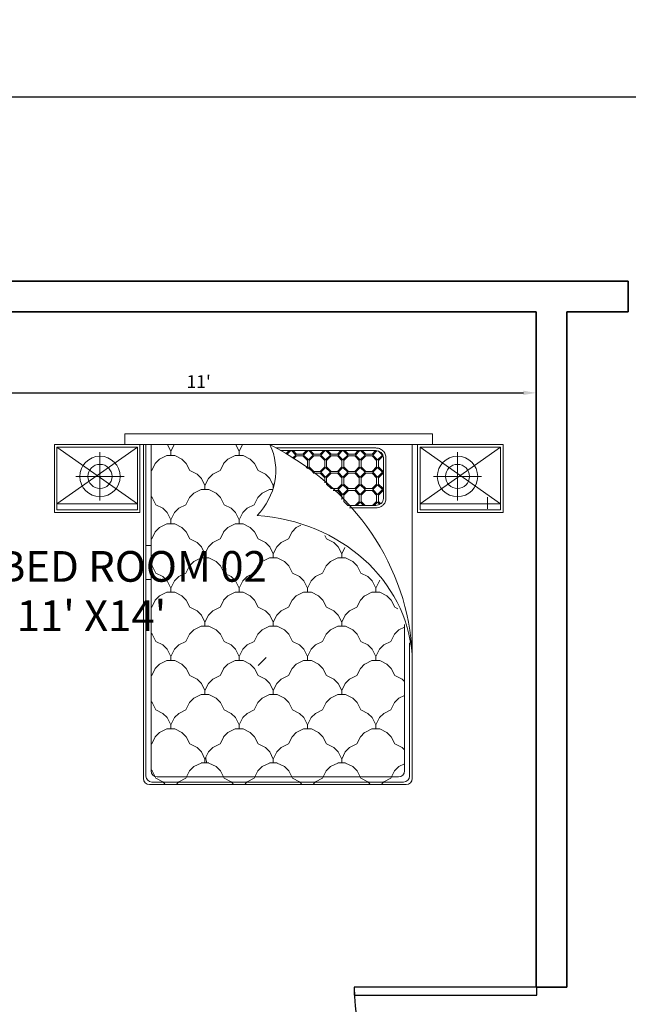
# Model space of a CAD drawing. Units: inches. Extents: x 2025 to 2528, y 1525 to 2336.
# Tile 7 of 18: x 2106 to 2225, y 1974 to 2167. Entities that reach past the tile are written whole.
import ezdxf

# ---------------------------------------------------------------- set-up
doc = ezdxf.new("R2010")
doc.units = ezdxf.units.IN
for name, color, linetype, lineweight in [('A-ANNO-DIMS', 2, 'Continuous', 18), ('A-AREA-IDEN', 7, 'Continuous', 25), ('A-DOOR', 3, 'Continuous', 25), ('A-FURN', 8, 'Continuous', 18), ('A-WALL', 7, 'Continuous', 35)]:
    doc.layers.add(name, color=color, linetype=linetype, lineweight=lineweight)
doc.styles.get("Standard").update_dxf_attribs({"font": 'arial.ttf'})
doc.dimstyles.new('Copy of ISO-25', dxfattribs={"dimtxt": 2.5, "dimasz": 2.5, "dimexe": 1.25, "dimexo": 0.625, "dimtad": 1, "dimdec": 1, "dimlunit": 4, "dimtxsty": 'Standard', "dimcen": 2.5, "dimadec": 0, "dimazin": 0, "dimtfac": 1, "dimtdec": 1, "dimtmove": 0, "dimatfit": 3, "dimfxl": 1, "dimarcsym": 0})

# ---------------------------------------------------------------- blocks, each defined once
blk = doc.blocks.new('*U5')
for p, q in [((0, 0), (0, -6)), ((-40, 0), (-40, -6))]:
    blk.add_line(p, q)
blk.add_lwpolyline([(0, 0), (0, 40), (-1.75, 40), (-1.75, 0)], close=True)
blk.add_arc((0, 0), 40, 90, 180)
blk = doc.blocks.new('*D12')
at = {"layer": 'A-ANNO-DIMS', "color": 0, "lineweight": -2, "transparency": 16777216}
for p, q in [((2075.01, 2108.79), (2075.01, 2092.35)), ((2207.01, 2108.79), (2207.01, 2092.35)), ((2077.51, 2093.6), (2204.51, 2093.6))]:
    blk.add_line(p, q, dxfattribs=at)
at = {"layer": 'A-ANNO-DIMS', "color": 0, "transparency": 16777216}
for points in [[(2077.51, 2094.02), (2077.51, 2093.19), (2075.01, 2093.6)], [(2204.51, 2094.02), (2204.51, 2093.19), (2207.01, 2093.6)]]:
    blk.add_solid(points, dxfattribs=at)
at = {"layer": 'Defpoints', "color": 0, "transparency": 16777216}
for p in [(2075.01, 2109.41), (2207.01, 2109.41), (2207.01, 2093.6)]:
    blk.add_point(p, dxfattribs=at)
at = {"layer": 'A-ANNO-DIMS', "color": 0, "transparency": 16777216, "insert": (2141.01, 2095.48), "char_height": 2.5, "attachment_point": 5}
blk.add_mtext("11'", dxfattribs=at)
blk = doc.blocks.new('A$C029D5C69')
for p, q in [((0.4164, 2.0693), (0.4164, 2.0066)), ((2.2315, 2.0693), (0.4164, 2.0693)), ((2.2315, 2.0066), (2.2315, 2.0693)), ((0, 1.606), (0, 2.0066)), ((0, 2.0066), (0.505, 2.0066)), ((0.0151, 1.6211), (0.0151, 1.9915)), ((0.0151, 1.9915), (0.4899, 1.9915)), ((0.4164, 2.0066), (2.2315, 2.0066)), ((0.4899, 1.9915), (0.4899, 1.6211)), ((0.505, 2.0066), (0.505, 1.606)), ((0.5252, 0.0351), (0.5252, 2.0066)), ((0.5403, 0.0502), (0.5403, 2.0066)), ((0.5706, 0.0805), (0.5706, 2.0066)), ((0.6869, 1.966), (0.6666, 2.0066)), ((0.7072, 2.0066), (0.6869, 1.966)), ((1.0902, 1.966), (1.0699, 2.0066)), ((1.1106, 2.0066), (1.0902, 1.966)), ((1.8954, 1.9865), (1.3081, 1.9865)), ((2.1114, 2.0087), (2.1114, 0.0351)), ((2.6479, 2.0066), (2.1429, 2.0066)), ((2.1429, 2.0066), (2.1429, 1.606)), ((2.6328, 1.9915), (2.158, 1.9915)), ((2.158, 1.9915), (2.158, 1.6211)), ((2.6328, 1.6211), (2.6328, 1.9915)), ((2.6479, 1.606), (2.6479, 2.0066)), ((0.2689, 1.9609), (0.2689, 1.6764)), ((0.621, 1.9213), (0.5955, 1.8958)), ((0.6634, 1.9425), (0.621, 1.9213)), ((0.6634, 1.9425), (0.621, 1.9213)), ((0.6869, 1.9425), (0.6634, 1.9425)), ((0.6869, 1.9425), (0.6869, 1.966)), ((0.6869, 1.9425), (0.6869, 1.966)), ((0.6869, 1.9425), (0.7104, 1.9425)), ((0.7528, 1.9213), (0.7104, 1.9425)), ((0.7528, 1.9213), (0.7104, 1.9425)), ((0.7783, 1.8958), (0.7528, 1.9213)), ((1.0243, 1.9213), (0.9988, 1.8958)), ((1.0668, 1.9425), (1.0244, 1.9213)), ((1.0668, 1.9425), (1.0244, 1.9213)), ((1.0902, 1.9425), (1.0668, 1.9425)), ((1.0902, 1.9425), (1.0902, 1.966)), ((1.0902, 1.9425), (1.0902, 1.966)), ((1.0902, 1.9425), (1.1137, 1.9425)), ((1.1561, 1.9213), (1.1137, 1.9425)), ((1.1561, 1.9213), (1.1137, 1.9425)), ((1.1816, 1.8958), (1.1561, 1.9213)), ((1.8954, 1.9713), (1.3339, 1.9713)), ((1.3849, 1.9713), (1.3656, 1.952)), ((1.3945, 1.9713), (1.3714, 1.9483)), ((1.4249, 1.945), (1.3986, 1.9713)), ((1.4249, 1.945), (1.4059, 1.926)), ((1.4288, 1.9507), (1.4081, 1.9713)), ((1.4288, 1.9394), (1.4116, 1.9222)), ((1.4476, 1.9507), (1.4288, 1.9507)), ((1.4288, 1.9393), (1.4476, 1.9393)), ((1.4476, 1.9507), (1.4664, 1.9507)), ((1.4664, 1.9393), (1.4476, 1.9393)), ((1.487, 1.9713), (1.4664, 1.9507)), ((1.493, 1.9128), (1.4664, 1.9394)), ((1.4966, 1.9713), (1.4703, 1.945)), ((1.4986, 1.9167), (1.4703, 1.945)), ((1.527, 1.945), (1.4986, 1.9167)), ((1.527, 1.945), (1.5007, 1.9713)), ((1.5309, 1.9394), (1.5043, 1.9128)), ((1.5309, 1.9507), (1.5102, 1.9713)), ((1.5497, 1.9507), (1.5309, 1.9507)), ((1.5309, 1.9393), (1.5497, 1.9393)), ((1.5497, 1.9507), (1.5685, 1.9507)), ((1.5685, 1.9393), (1.5497, 1.9393)), ((1.5891, 1.9713), (1.5685, 1.9507)), ((1.595, 1.9128), (1.5685, 1.9394)), ((1.5987, 1.9713), (1.5724, 1.945)), ((1.6007, 1.9167), (1.5724, 1.945)), ((1.6291, 1.945), (1.6007, 1.9167)), ((1.6291, 1.945), (1.6028, 1.9713)), ((1.633, 1.9394), (1.6064, 1.9128)), ((1.633, 1.9507), (1.6123, 1.9713)), ((1.6518, 1.9507), (1.633, 1.9507)), ((1.633, 1.9393), (1.6518, 1.9393)), ((1.6518, 1.9507), (1.6706, 1.9507)), ((1.6706, 1.9393), (1.6518, 1.9393)), ((1.6912, 1.9713), (1.6706, 1.9507)), ((1.6971, 1.9128), (1.6706, 1.9394)), ((1.7008, 1.9713), (1.6745, 1.945)), ((1.7028, 1.9167), (1.6745, 1.945)), ((1.7312, 1.945), (1.7028, 1.9167)), ((1.7312, 1.945), (1.7049, 1.9713)), ((1.7351, 1.9394), (1.7085, 1.9128)), ((1.7351, 1.9507), (1.7144, 1.9713)), ((1.7539, 1.9507), (1.7351, 1.9507)), ((1.7351, 1.9393), (1.7539, 1.9393)), ((1.7539, 1.9507), (1.7727, 1.9507)), ((1.7727, 1.9393), (1.7539, 1.9393)), ((1.7933, 1.9713), (1.7727, 1.9507)), ((1.7992, 1.9128), (1.7727, 1.9394)), ((1.8029, 1.9713), (1.7766, 1.945)), ((1.8049, 1.9167), (1.7766, 1.945)), ((1.8333, 1.945), (1.8049, 1.9167)), ((1.8333, 1.945), (1.807, 1.9713)), ((1.8372, 1.9394), (1.8106, 1.9128)), ((1.8372, 1.9507), (1.8165, 1.9713)), ((1.856, 1.9507), (1.8372, 1.9507)), ((1.8372, 1.9393), (1.856, 1.9393)), ((1.856, 1.9507), (1.8748, 1.9507)), ((1.8748, 1.9393), (1.856, 1.9393)), ((1.8954, 1.9713), (1.8748, 1.9507)), ((1.9013, 1.9128), (1.8748, 1.9394)), ((1.9043, 1.9707), (1.8787, 1.945)), ((1.907, 1.9167), (1.8787, 1.945)), ((1.9354, 1.945), (1.907, 1.9167)), ((1.9354, 1.945), (1.9114, 1.969)), ((1.9393, 1.9394), (1.9127, 1.9128)), ((1.9393, 1.9393), (1.9404, 1.9393)), ((1.9414, 1.688), (1.9414, 1.931)), ((1.9565, 1.688), (1.9565, 1.931)), ((2.379, 1.9609), (2.379, 1.6764)), ((0.5955, 1.8958), (0.5743, 1.8534)), ((0.7995, 1.8534), (0.7783, 1.8958)), ((0.9989, 1.8958), (0.9777, 1.8534)), ((1.2028, 1.8534), (1.1816, 1.8958)), ((1.493, 1.8752), (1.4867, 1.869)), ((1.4986, 1.8713), (1.4922, 1.8648)), ((1.493, 1.8752), (1.493, 1.9128)), ((1.527, 1.8429), (1.4986, 1.8713)), ((1.5043, 1.8752), (1.5043, 1.9128)), ((1.5309, 1.8486), (1.5043, 1.8752)), ((1.595, 1.8752), (1.5685, 1.8486)), ((1.6007, 1.8713), (1.5724, 1.8429)), ((1.595, 1.8752), (1.595, 1.9128)), ((1.6291, 1.8429), (1.6007, 1.8713)), ((1.6064, 1.8752), (1.6064, 1.9128)), ((1.633, 1.8486), (1.6064, 1.8752)), ((1.6971, 1.8752), (1.6706, 1.8486)), ((1.7028, 1.8713), (1.6745, 1.8429)), ((1.6971, 1.8752), (1.6971, 1.9128)), ((1.7312, 1.8429), (1.7028, 1.8713)), ((1.7085, 1.8752), (1.7085, 1.9128)), ((1.7351, 1.8486), (1.7085, 1.8752)), ((1.7992, 1.8752), (1.7727, 1.8486)), ((1.8049, 1.8713), (1.7766, 1.8429)), ((1.7992, 1.8752), (1.7992, 1.9128)), ((1.8333, 1.8429), (1.8049, 1.8713)), ((1.8106, 1.8752), (1.8106, 1.9128)), ((1.8372, 1.8486), (1.8106, 1.8752)), ((1.9013, 1.8752), (1.8748, 1.8486)), ((1.907, 1.8713), (1.8787, 1.8429)), ((1.9013, 1.8752), (1.9013, 1.9128)), ((1.9354, 1.8429), (1.907, 1.8713)), ((1.9127, 1.8752), (1.9127, 1.9128)), ((1.9393, 1.8486), (1.9127, 1.8752)), ((0.1267, 1.8186), (0.4111, 1.8186)), ((0.5743, 1.8534), (0.5706, 1.8515)), ((0.5743, 1.8534), (0.5706, 1.8515)), ((0.8419, 1.8322), (0.7995, 1.8534)), ((0.8419, 1.8322), (0.7995, 1.8534)), ((0.8674, 1.8067), (0.8419, 1.8322)), ((0.8886, 1.7643), (0.8674, 1.8067)), ((0.9098, 1.8067), (0.8886, 1.7643)), ((0.9352, 1.8322), (0.9097, 1.8067)), ((0.9777, 1.8534), (0.9353, 1.8322)), ((0.9777, 1.8534), (0.9353, 1.8322)), ((1.2452, 1.8322), (1.2028, 1.8534)), ((1.2452, 1.8322), (1.2028, 1.8534)), ((1.2707, 1.8067), (1.2452, 1.8322)), ((1.2919, 1.7643), (1.2707, 1.8067)), ((1.527, 1.8429), (1.5242, 1.8401)), ((1.5309, 1.8373), (1.5295, 1.8359)), ((1.5497, 1.8486), (1.5309, 1.8486)), ((1.5309, 1.8373), (1.5497, 1.8373)), ((1.5497, 1.8486), (1.5685, 1.8486)), ((1.5685, 1.8373), (1.5497, 1.8373)), ((1.595, 1.8107), (1.5685, 1.8373)), ((1.6007, 1.8146), (1.5724, 1.8429)), ((1.595, 1.7806), (1.595, 1.8107)), ((1.6291, 1.8429), (1.6007, 1.8146)), ((1.633, 1.8373), (1.6064, 1.8107)), ((1.6064, 1.7731), (1.6064, 1.8107)), ((1.6518, 1.8486), (1.633, 1.8486)), ((1.633, 1.8373), (1.6518, 1.8373)), ((1.6518, 1.8486), (1.6706, 1.8486)), ((1.6706, 1.8373), (1.6518, 1.8373)), ((1.6971, 1.8107), (1.6706, 1.8373)), ((1.7028, 1.8146), (1.6745, 1.8429)), ((1.6971, 1.7731), (1.6971, 1.8107)), ((1.7312, 1.8429), (1.7028, 1.8146)), ((1.7351, 1.8373), (1.7085, 1.8107)), ((1.7085, 1.7731), (1.7085, 1.8107)), ((1.7539, 1.8486), (1.7351, 1.8486)), ((1.7351, 1.8373), (1.7539, 1.8373)), ((1.7539, 1.8486), (1.7727, 1.8486)), ((1.7727, 1.8373), (1.7539, 1.8373)), ((1.7992, 1.8107), (1.7727, 1.8373)), ((1.8049, 1.8146), (1.7766, 1.8429)), ((1.7992, 1.7731), (1.7992, 1.8107)), ((1.8333, 1.8429), (1.8049, 1.8146)), ((1.8372, 1.8373), (1.8106, 1.8107)), ((1.8106, 1.7731), (1.8106, 1.8107)), ((1.856, 1.8486), (1.8372, 1.8486)), ((1.8372, 1.8373), (1.856, 1.8373)), ((1.856, 1.8486), (1.8748, 1.8486)), ((1.8748, 1.8373), (1.856, 1.8373)), ((1.9013, 1.8107), (1.8748, 1.8373)), ((1.907, 1.8146), (1.8787, 1.8429)), ((1.9013, 1.7731), (1.9013, 1.8107)), ((1.9354, 1.8429), (1.907, 1.8146)), ((1.9393, 1.8373), (1.9127, 1.8107)), ((1.9127, 1.7731), (1.9127, 1.8107)), ((1.9414, 1.8486), (1.9393, 1.8486)), ((1.9393, 1.8373), (1.9414, 1.8373)), ((2.2367, 1.8186), (2.5212, 1.8186)), ((0.8886, 1.7408), (0.8886, 1.7643)), ((1.2981, 1.7768), (1.2919, 1.7643)), ((1.2919, 1.7519), (1.2919, 1.7643)), ((1.633, 1.7465), (1.6064, 1.7731)), ((1.6518, 1.7465), (1.633, 1.7465)), ((1.6518, 1.7465), (1.6706, 1.7465)), ((1.6971, 1.7731), (1.6706, 1.7465)), ((1.7028, 1.7692), (1.6745, 1.7408)), ((1.7312, 1.7408), (1.7028, 1.7692)), ((1.7351, 1.7465), (1.7085, 1.7731)), ((1.7539, 1.7465), (1.7351, 1.7465)), ((1.7539, 1.7465), (1.7727, 1.7465)), ((1.7992, 1.7731), (1.7727, 1.7465)), ((1.8049, 1.7692), (1.7766, 1.7408)), ((1.8333, 1.7408), (1.8049, 1.7692)), ((1.8372, 1.7465), (1.8106, 1.7731)), ((1.856, 1.7465), (1.8372, 1.7465)), ((1.856, 1.7465), (1.8748, 1.7465)), ((1.9013, 1.7731), (1.8748, 1.7465)), ((1.907, 1.7692), (1.8787, 1.7408)), ((1.9354, 1.7408), (1.907, 1.7692)), ((1.9393, 1.7465), (1.9127, 1.7731)), ((1.9414, 1.7465), (1.9393, 1.7465)), ((0.5766, 1.6941), (0.5706, 1.7002)), ((0.5978, 1.6517), (0.5766, 1.6941)), ((0.7972, 1.6941), (0.776, 1.6517)), ((0.8227, 1.7196), (0.7972, 1.6941)), ((0.8651, 1.7408), (0.8227, 1.7196)), ((0.8651, 1.7408), (0.8227, 1.7196)), ((0.912, 1.7408), (0.8651, 1.7408)), ((0.9544, 1.7196), (0.912, 1.7408)), ((0.9544, 1.7196), (0.912, 1.7408)), ((0.98, 1.6941), (0.9545, 1.7196)), ((1.0011, 1.6517), (0.9799, 1.6941)), ((1.2005, 1.6941), (1.1793, 1.6517)), ((1.226, 1.7196), (1.2005, 1.6941)), ((1.2684, 1.7408), (1.226, 1.7196)), ((1.2684, 1.7408), (1.226, 1.7196)), ((1.2885, 1.7408), (1.2684, 1.7408)), ((1.6443, 1.7352), (1.6518, 1.7352)), ((1.6706, 1.7352), (1.6518, 1.7352)), ((1.6971, 1.7086), (1.6706, 1.7352)), ((1.7028, 1.7125), (1.6745, 1.7408)), ((1.6971, 1.682), (1.6971, 1.7086)), ((1.7312, 1.7408), (1.7028, 1.7125)), ((1.7351, 1.7352), (1.7085, 1.7086)), ((1.7085, 1.671), (1.7085, 1.7086)), ((1.7351, 1.7352), (1.7539, 1.7352)), ((1.7727, 1.7352), (1.7539, 1.7352)), ((1.7992, 1.7086), (1.7727, 1.7352)), ((1.8049, 1.7125), (1.7766, 1.7408)), ((1.7992, 1.671), (1.7992, 1.7086)), ((1.8333, 1.7408), (1.8049, 1.7125)), ((1.8372, 1.7352), (1.8106, 1.7086)), ((1.8106, 1.671), (1.8106, 1.7086)), ((1.8372, 1.7352), (1.856, 1.7352)), ((1.8748, 1.7352), (1.856, 1.7352)), ((1.9013, 1.7086), (1.8748, 1.7352)), ((1.907, 1.7125), (1.8787, 1.7408)), ((1.9013, 1.671), (1.9013, 1.7086)), ((1.9354, 1.7408), (1.907, 1.7125)), ((1.9393, 1.7352), (1.9127, 1.7086)), ((1.9127, 1.671), (1.9127, 1.7086)), ((1.9393, 1.7352), (1.9414, 1.7352)), ((2.5551, 1.6275), (2.5551, 1.696)), ((0.6402, 1.6305), (0.5978, 1.6517)), ((0.6402, 1.6305), (0.5978, 1.6517)), ((0.6657, 1.605), (0.6402, 1.6305)), ((0.7336, 1.6305), (0.7081, 1.605)), ((0.776, 1.6517), (0.7336, 1.6305)), ((0.776, 1.6517), (0.7336, 1.6305)), ((1.0435, 1.6305), (1.0011, 1.6517)), ((1.0435, 1.6305), (1.0011, 1.6517)), ((1.0691, 1.605), (1.0436, 1.6305)), ((1.1369, 1.6305), (1.1114, 1.605)), ((1.1793, 1.6517), (1.1369, 1.6305)), ((1.1793, 1.6517), (1.1369, 1.6305)), ((1.7318, 1.6477), (1.7085, 1.671)), ((1.8961, 1.6477), (1.7289, 1.6477)), ((1.8961, 1.6325), (1.7422, 1.6325)), ((1.7992, 1.671), (1.7759, 1.6477)), ((1.8049, 1.6671), (1.7855, 1.6477)), ((1.8244, 1.6477), (1.8049, 1.6671)), ((1.8339, 1.6477), (1.8106, 1.671)), ((1.9013, 1.671), (1.878, 1.6477)), ((1.907, 1.6671), (1.8876, 1.6477)), ((1.9202, 1.6539), (1.907, 1.6671)), ((1.926, 1.6577), (1.9127, 1.671)), ((0.505, 1.606), (0, 1.606)), ((0.4899, 1.6211), (0.0151, 1.6211)), ((0.6869, 1.5626), (0.6657, 1.605)), ((0.7081, 1.605), (0.6869, 1.5626)), ((1.0902, 1.5626), (1.069, 1.605)), ((1.1114, 1.605), (1.0902, 1.5626)), ((2.1429, 1.606), (2.6479, 1.606)), ((2.158, 1.6211), (2.6328, 1.6211)), ((0.621, 1.5179), (0.5955, 1.4924)), ((0.6634, 1.5391), (0.621, 1.5179)), ((0.6634, 1.5391), (0.621, 1.5179)), ((0.6869, 1.5392), (0.6634, 1.5392)), ((0.6869, 1.5392), (0.6869, 1.5626)), ((0.6869, 1.5392), (0.6869, 1.5626)), ((0.6869, 1.5392), (0.7104, 1.5392)), ((0.7528, 1.5179), (0.7104, 1.5391)), ((0.7528, 1.5179), (0.7104, 1.5391)), ((0.7783, 1.4924), (0.7528, 1.5179)), ((1.0243, 1.5179), (0.9988, 1.4924)), ((1.0668, 1.5391), (1.0244, 1.5179)), ((1.0668, 1.5391), (1.0244, 1.5179)), ((1.0902, 1.5392), (1.0668, 1.5392)), ((1.0902, 1.5392), (1.0902, 1.5626)), ((1.0902, 1.5392), (1.0902, 1.5626)), ((1.0902, 1.5392), (1.1137, 1.5392)), ((1.1561, 1.5179), (1.1137, 1.5391)), ((1.1561, 1.5179), (1.1137, 1.5391)), ((1.1816, 1.4924), (1.1561, 1.5179)), ((1.4277, 1.5179), (1.4022, 1.4924)), ((1.4534, 1.5308), (1.4277, 1.5179)), ((1.4534, 1.5308), (1.4277, 1.5179)), ((0.5955, 1.4925), (0.5743, 1.4501)), ((0.7995, 1.4501), (0.7783, 1.4925)), ((0.9989, 1.4925), (0.9777, 1.4501)), ((1.2028, 1.4501), (1.1816, 1.4925)), ((1.4022, 1.4925), (1.381, 1.4501)), ((1.6062, 1.4501), (1.5966, 1.4692)), ((0.5403, 1.4117), (0.5706, 1.4117)), ((0.5743, 1.45), (0.5706, 1.4481)), ((0.5743, 1.45), (0.5706, 1.4481)), ((0.8419, 1.4288), (0.7995, 1.45)), ((0.8419, 1.4288), (0.7995, 1.45)), ((0.8674, 1.4033), (0.8419, 1.4288)), ((0.8886, 1.361), (0.8674, 1.4034)), ((0.9098, 1.4034), (0.8886, 1.361)), ((0.9352, 1.4288), (0.9097, 1.4033)), ((0.9777, 1.45), (0.9353, 1.4288)), ((0.9777, 1.45), (0.9353, 1.4288)), ((1.2452, 1.4288), (1.2028, 1.45)), ((1.2452, 1.4288), (1.2028, 1.45)), ((1.2707, 1.4033), (1.2452, 1.4288)), ((1.2919, 1.361), (1.2707, 1.4034)), ((1.3131, 1.4034), (1.2919, 1.361)), ((1.3386, 1.4288), (1.3131, 1.4033)), ((1.381, 1.45), (1.3386, 1.4288)), ((1.381, 1.45), (1.3386, 1.4288)), ((1.6486, 1.4288), (1.6062, 1.45)), ((1.6486, 1.4288), (1.6062, 1.45)), ((1.6741, 1.4033), (1.6486, 1.4288)), ((1.6953, 1.361), (1.6741, 1.4034)), ((1.714, 1.3984), (1.6953, 1.361)), ((0.8651, 1.3374), (0.8227, 1.3162)), ((0.8651, 1.3374), (0.8227, 1.3162)), ((0.912, 1.3375), (0.8651, 1.3375)), ((0.8886, 1.3375), (0.8886, 1.3609)), ((0.9544, 1.3162), (0.912, 1.3374)), ((0.9544, 1.3162), (0.912, 1.3374)), ((1.2684, 1.3374), (1.226, 1.3162)), ((1.2684, 1.3374), (1.226, 1.3162)), ((1.3154, 1.3375), (1.2684, 1.3375)), ((1.2919, 1.3375), (1.2919, 1.3609)), ((1.3578, 1.3162), (1.3154, 1.3374)), ((1.3578, 1.3162), (1.3154, 1.3374)), ((1.6718, 1.3374), (1.6294, 1.3162)), ((1.6718, 1.3374), (1.6294, 1.3162)), ((1.7187, 1.3375), (1.6718, 1.3375)), ((1.6953, 1.3375), (1.6953, 1.3609)), ((1.7611, 1.3162), (1.7187, 1.3374)), ((1.7611, 1.3162), (1.7187, 1.3374)), ((0.5766, 1.2908), (0.5706, 1.2968)), ((0.5978, 1.2484), (0.5766, 1.2908)), ((0.7972, 1.2908), (0.776, 1.2484)), ((0.8227, 1.3163), (0.7972, 1.2908)), ((0.98, 1.2908), (0.9545, 1.3163)), ((1.0011, 1.2484), (0.9799, 1.2908)), ((1.2005, 1.2908), (1.1793, 1.2484)), ((1.226, 1.3163), (1.2005, 1.2908)), ((1.3833, 1.2908), (1.3578, 1.3163)), ((1.4045, 1.2484), (1.3833, 1.2908)), ((1.6039, 1.2908), (1.5827, 1.2484)), ((1.6294, 1.3163), (1.6039, 1.2908)), ((1.7867, 1.2908), (1.7611, 1.3163)), ((1.8078, 1.2484), (1.7866, 1.2908)), ((0.6402, 1.2271), (0.5978, 1.2483)), ((0.6402, 1.2271), (0.5978, 1.2483)), ((0.6657, 1.2017), (0.6402, 1.2272)), ((0.7336, 1.2272), (0.7081, 1.2017)), ((0.776, 1.2483), (0.7336, 1.2271)), ((0.776, 1.2483), (0.7336, 1.2271)), ((1.0435, 1.2271), (1.0011, 1.2483)), ((1.0435, 1.2271), (1.0011, 1.2483)), ((1.0691, 1.2017), (1.0436, 1.2272)), ((1.1369, 1.2272), (1.1114, 1.2017)), ((1.1793, 1.2483), (1.1369, 1.2271)), ((1.1793, 1.2483), (1.1369, 1.2271)), ((1.4469, 1.2271), (1.4045, 1.2483)), ((1.4469, 1.2271), (1.4045, 1.2483)), ((1.4724, 1.2017), (1.4469, 1.2272)), ((1.5403, 1.2272), (1.5148, 1.2017)), ((1.5827, 1.2483), (1.5403, 1.2271)), ((1.5827, 1.2483), (1.5403, 1.2271)), ((1.8502, 1.2271), (1.8078, 1.2483)), ((1.8502, 1.2271), (1.8078, 1.2483)), ((1.8758, 1.2017), (1.8503, 1.2272)), ((0.5403, 1.21), (0.5706, 1.21)), ((0.6869, 1.1593), (0.6657, 1.2017)), ((0.7081, 1.2017), (0.6869, 1.1593)), ((1.0902, 1.1593), (1.069, 1.2017)), ((1.1114, 1.2017), (1.0902, 1.1593)), ((1.4936, 1.1593), (1.4724, 1.2017)), ((1.5148, 1.2017), (1.4936, 1.1593)), ((1.8969, 1.1593), (1.8757, 1.2017)), ((1.9181, 1.2017), (1.8969, 1.1593)), ((1.9215, 1.2051), (1.9181, 1.2017)), ((0.621, 1.1146), (0.5955, 1.0891)), ((0.6634, 1.1358), (0.621, 1.1146)), ((0.6634, 1.1358), (0.621, 1.1146)), ((0.6869, 1.1358), (0.6634, 1.1358)), ((0.6869, 1.1358), (0.6869, 1.1593)), ((0.6869, 1.1358), (0.6869, 1.1593)), ((0.6869, 1.1358), (0.7104, 1.1358)), ((0.7528, 1.1146), (0.7104, 1.1358)), ((0.7528, 1.1146), (0.7104, 1.1358)), ((0.7783, 1.0891), (0.7528, 1.1146)), ((1.0243, 1.1146), (0.9988, 1.0891)), ((1.0668, 1.1358), (1.0244, 1.1146)), ((1.0668, 1.1358), (1.0244, 1.1146)), ((1.0902, 1.1358), (1.0668, 1.1358)), ((1.0902, 1.1358), (1.0902, 1.1593)), ((1.0902, 1.1358), (1.0902, 1.1593)), ((1.0902, 1.1358), (1.1137, 1.1358)), ((1.1561, 1.1146), (1.1137, 1.1358)), ((1.1561, 1.1146), (1.1137, 1.1358)), ((1.1816, 1.0891), (1.1561, 1.1146)), ((1.4277, 1.1146), (1.4022, 1.0891)), ((1.4701, 1.1358), (1.4277, 1.1146)), ((1.4701, 1.1358), (1.4277, 1.1146)), ((1.4936, 1.1358), (1.4701, 1.1358)), ((1.4936, 1.1358), (1.4936, 1.1593)), ((1.4936, 1.1358), (1.4936, 1.1593)), ((1.4936, 1.1358), (1.5171, 1.1358)), ((1.5595, 1.1146), (1.5171, 1.1358)), ((1.5595, 1.1146), (1.5171, 1.1358)), ((1.585, 1.0891), (1.5595, 1.1146)), ((1.831, 1.1146), (1.8055, 1.0891)), ((1.8735, 1.1358), (1.8311, 1.1146)), ((1.8735, 1.1358), (1.8311, 1.1146)), ((1.8969, 1.1358), (1.8735, 1.1358)), ((1.8969, 1.1358), (1.8969, 1.1593)), ((1.8969, 1.1358), (1.8969, 1.1593)), ((1.8969, 1.1358), (1.9204, 1.1358)), ((1.9628, 1.1146), (1.9204, 1.1358)), ((1.9628, 1.1146), (1.9204, 1.1358)), ((1.9883, 1.0891), (1.9628, 1.1146)), ((0.5743, 1.0467), (0.5706, 1.0448)), ((0.5743, 1.0467), (0.5706, 1.0448)), ((0.5955, 1.0891), (0.5743, 1.0467)), ((0.7995, 1.0467), (0.7783, 1.0891)), ((0.8419, 1.0255), (0.7995, 1.0467)), ((0.8419, 1.0255), (0.7995, 1.0467)), ((0.9777, 1.0467), (0.9353, 1.0255)), ((0.9777, 1.0467), (0.9353, 1.0255)), ((0.9989, 1.0891), (0.9777, 1.0467)), ((1.2028, 1.0467), (1.1816, 1.0891)), ((1.2452, 1.0255), (1.2028, 1.0467)), ((1.2452, 1.0255), (1.2028, 1.0467)), ((1.381, 1.0467), (1.3386, 1.0255)), ((1.381, 1.0467), (1.3386, 1.0255)), ((1.4022, 1.0891), (1.381, 1.0467)), ((1.6062, 1.0467), (1.585, 1.0891)), ((1.6486, 1.0255), (1.6062, 1.0467)), ((1.6486, 1.0255), (1.6062, 1.0467)), ((1.7844, 1.0467), (1.742, 1.0255)), ((1.7844, 1.0467), (1.742, 1.0255)), ((1.8056, 1.0891), (1.7844, 1.0467)), ((2.0095, 1.0467), (1.9883, 1.0891)), ((2.0276, 1.0376), (2.0095, 1.0467)), ((2.0276, 1.0376), (2.0095, 1.0467)), ((0.8674, 1), (0.8419, 1.0255)), ((0.8886, 0.9576), (0.8674, 1)), ((0.9098, 1), (0.8886, 0.9576)), ((0.9352, 1.0255), (0.9097, 1)), ((1.2707, 1), (1.2452, 1.0255)), ((1.2919, 0.9576), (1.2707, 1)), ((1.3131, 1), (1.2919, 0.9576)), ((1.3386, 1.0255), (1.3131, 1)), ((1.6741, 1), (1.6486, 1.0255)), ((1.6953, 0.9576), (1.6741, 1)), ((1.7165, 1), (1.6953, 0.9576)), ((1.7419, 1.0255), (1.7164, 1)), ((0.8651, 0.9341), (0.8227, 0.9129)), ((0.8651, 0.9341), (0.8227, 0.9129)), ((0.912, 0.9341), (0.8651, 0.9341)), ((0.8886, 0.9341), (0.8886, 0.9576)), ((0.9544, 0.9129), (0.912, 0.9341)), ((0.9544, 0.9129), (0.912, 0.9341)), ((1.2684, 0.9341), (1.226, 0.9129)), ((1.2684, 0.9341), (1.226, 0.9129)), ((1.3154, 0.9341), (1.2684, 0.9341)), ((1.2919, 0.9341), (1.2919, 0.9576)), ((1.3578, 0.9129), (1.3154, 0.9341)), ((1.3578, 0.9129), (1.3154, 0.9341)), ((1.6718, 0.9341), (1.6294, 0.9129)), ((1.6718, 0.9341), (1.6294, 0.9129)), ((1.7187, 0.9341), (1.6718, 0.9341)), ((1.6953, 0.9341), (1.6953, 0.9576)), ((1.7611, 0.9129), (1.7187, 0.9341)), ((1.7611, 0.9129), (1.7187, 0.9341)), ((2.066, 0.9457), (2.066, 0.0805)), ((0.5766, 0.8874), (0.5706, 0.8935)), ((0.5978, 0.845), (0.5766, 0.8874)), ((0.7972, 0.8874), (0.776, 0.845)), ((0.8227, 0.9129), (0.7972, 0.8874)), ((0.98, 0.8874), (0.9545, 0.9129)), ((1.0011, 0.845), (0.9799, 0.8874)), ((1.2005, 0.8874), (1.1793, 0.845)), ((1.226, 0.9129), (1.2005, 0.8874)), ((1.3833, 0.8874), (1.3578, 0.9129)), ((1.4045, 0.845), (1.3833, 0.8874)), ((1.6039, 0.8874), (1.5827, 0.845)), ((1.6294, 0.9129), (1.6039, 0.8874)), ((1.7867, 0.8874), (1.7611, 0.9129)), ((1.8078, 0.845), (1.7866, 0.8874)), ((2.0072, 0.8874), (1.986, 0.845)), ((2.0327, 0.9129), (2.0072, 0.8874)), ((2.066, 0.9295), (2.0327, 0.9129)), ((2.066, 0.9295), (2.0327, 0.9129)), ((0.6402, 0.8238), (0.5978, 0.845)), ((0.6402, 0.8238), (0.5978, 0.845)), ((0.6657, 0.7983), (0.6402, 0.8238)), ((0.7336, 0.8238), (0.7081, 0.7983)), ((0.776, 0.845), (0.7336, 0.8238)), ((0.776, 0.845), (0.7336, 0.8238)), ((1.0435, 0.8238), (1.0011, 0.845)), ((1.0435, 0.8238), (1.0011, 0.845)), ((1.0691, 0.7983), (1.0436, 0.8238)), ((1.1369, 0.8238), (1.1114, 0.7983)), ((1.1793, 0.845), (1.1369, 0.8238)), ((1.1793, 0.845), (1.1369, 0.8238)), ((1.4469, 0.8238), (1.4045, 0.845)), ((1.4469, 0.8238), (1.4045, 0.845)), ((1.4724, 0.7983), (1.4469, 0.8238)), ((1.5403, 0.8238), (1.5148, 0.7983)), ((1.5827, 0.845), (1.5403, 0.8238)), ((1.5827, 0.845), (1.5403, 0.8238)), ((1.8502, 0.8238), (1.8078, 0.845)), ((1.8502, 0.8238), (1.8078, 0.845)), ((1.8758, 0.7983), (1.8503, 0.8238)), ((1.9436, 0.8238), (1.9181, 0.7983)), ((1.986, 0.845), (1.9436, 0.8238)), ((1.986, 0.845), (1.9436, 0.8238)), ((2.0962, 0.8369), (2.0962, 0.0502)), ((0.6869, 0.7559), (0.6657, 0.7983)), ((0.7081, 0.7983), (0.6869, 0.7559)), ((0.6869, 0.7325), (0.6869, 0.7559)), ((0.6869, 0.7325), (0.6869, 0.7559)), ((1.0902, 0.7559), (1.069, 0.7983)), ((1.1114, 0.7983), (1.0902, 0.7559)), ((1.0902, 0.7325), (1.0902, 0.7559)), ((1.0902, 0.7325), (1.0902, 0.7559)), ((1.4936, 0.7559), (1.4724, 0.7983)), ((1.5148, 0.7983), (1.4936, 0.7559)), ((1.4936, 0.7325), (1.4936, 0.7559)), ((1.4936, 0.7325), (1.4936, 0.7559)), ((1.8969, 0.7559), (1.8757, 0.7983)), ((1.9181, 0.7983), (1.8969, 0.7559)), ((1.8969, 0.7325), (1.8969, 0.7559)), ((1.8969, 0.7325), (1.8969, 0.7559)), ((0.621, 0.7113), (0.5955, 0.6858)), ((0.6634, 0.7324), (0.621, 0.7112)), ((0.6634, 0.7324), (0.621, 0.7112)), ((0.6869, 0.7325), (0.6634, 0.7325)), ((0.6869, 0.7325), (0.7104, 0.7325)), ((0.7528, 0.7112), (0.7104, 0.7324)), ((0.7528, 0.7112), (0.7104, 0.7324)), ((0.7783, 0.6858), (0.7528, 0.7113)), ((1.0243, 0.7113), (0.9988, 0.6858)), ((1.0668, 0.7324), (1.0244, 0.7112)), ((1.0668, 0.7324), (1.0244, 0.7112)), ((1.0902, 0.7325), (1.0668, 0.7325)), ((1.0902, 0.7325), (1.1137, 0.7325)), ((1.1561, 0.7112), (1.1137, 0.7324)), ((1.1561, 0.7112), (1.1137, 0.7324)), ((1.1816, 0.6858), (1.1561, 0.7113)), ((1.2024, 0.7028), (1.2503, 0.7507)), ((1.4277, 0.7113), (1.4022, 0.6858)), ((1.4701, 0.7324), (1.4277, 0.7112)), ((1.4701, 0.7324), (1.4277, 0.7112)), ((1.4936, 0.7325), (1.4701, 0.7325)), ((1.4936, 0.7325), (1.5171, 0.7325)), ((1.5595, 0.7112), (1.5171, 0.7324)), ((1.5595, 0.7112), (1.5171, 0.7324)), ((1.585, 0.6858), (1.5595, 0.7113)), ((1.831, 0.7113), (1.8055, 0.6858)), ((1.8735, 0.7324), (1.8311, 0.7112)), ((1.8735, 0.7324), (1.8311, 0.7112)), ((1.8969, 0.7325), (1.8735, 0.7325)), ((1.8969, 0.7325), (1.9204, 0.7325)), ((1.9628, 0.7112), (1.9204, 0.7324)), ((1.9628, 0.7112), (1.9204, 0.7324)), ((1.9883, 0.6858), (1.9628, 0.7113)), ((0.5743, 0.6433), (0.5706, 0.6414)), ((0.5743, 0.6433), (0.5706, 0.6414)), ((0.5955, 0.6858), (0.5743, 0.6434)), ((0.7995, 0.6434), (0.7783, 0.6858)), ((0.8419, 0.6221), (0.7995, 0.6433)), ((0.8419, 0.6221), (0.7995, 0.6433)), ((0.9777, 0.6433), (0.9353, 0.6221)), ((0.9777, 0.6433), (0.9353, 0.6221)), ((0.9989, 0.6858), (0.9777, 0.6434)), ((1.2028, 0.6434), (1.1816, 0.6858)), ((1.2452, 0.6221), (1.2028, 0.6433)), ((1.2452, 0.6221), (1.2028, 0.6433)), ((1.381, 0.6433), (1.3386, 0.6221)), ((1.381, 0.6433), (1.3386, 0.6221)), ((1.4022, 0.6858), (1.381, 0.6434)), ((1.6062, 0.6434), (1.585, 0.6858)), ((1.6486, 0.6221), (1.6062, 0.6433)), ((1.6486, 0.6221), (1.6062, 0.6433)), ((1.7844, 0.6433), (1.742, 0.6221)), ((1.7844, 0.6433), (1.742, 0.6221)), ((1.8056, 0.6858), (1.7844, 0.6434)), ((2.0095, 0.6434), (1.9883, 0.6858)), ((2.0519, 0.6221), (2.0095, 0.6433)), ((2.0519, 0.6221), (2.0095, 0.6433)), ((0.8674, 0.5967), (0.8419, 0.6222)), ((0.8886, 0.5543), (0.8674, 0.5967)), ((0.9098, 0.5967), (0.8886, 0.5543)), ((0.9352, 0.6222), (0.9097, 0.5967)), ((1.2707, 0.5967), (1.2452, 0.6222)), ((1.2919, 0.5543), (1.2707, 0.5967)), ((1.3131, 0.5967), (1.2919, 0.5543)), ((1.3386, 0.6222), (1.3131, 0.5967)), ((1.6741, 0.5967), (1.6486, 0.6222)), ((1.6953, 0.5543), (1.6741, 0.5967)), ((1.7165, 0.5967), (1.6953, 0.5543)), ((1.7419, 0.6222), (1.7164, 0.5967)), ((2.066, 0.6081), (2.0519, 0.6222)), ((0.8651, 0.5308), (0.8227, 0.5096)), ((0.8651, 0.5308), (0.8227, 0.5096)), ((0.912, 0.5308), (0.8651, 0.5308)), ((0.8886, 0.5308), (0.8886, 0.5543)), ((0.9544, 0.5096), (0.912, 0.5308)), ((0.9544, 0.5096), (0.912, 0.5308)), ((1.2684, 0.5308), (1.226, 0.5096)), ((1.2684, 0.5308), (1.226, 0.5096)), ((1.3154, 0.5308), (1.2684, 0.5308)), ((1.2919, 0.5308), (1.2919, 0.5543)), ((1.3578, 0.5096), (1.3154, 0.5308)), ((1.3578, 0.5096), (1.3154, 0.5308)), ((1.6718, 0.5308), (1.6294, 0.5096)), ((1.6718, 0.5308), (1.6294, 0.5096)), ((1.7187, 0.5308), (1.6718, 0.5308)), ((1.6953, 0.5308), (1.6953, 0.5543)), ((1.7611, 0.5096), (1.7187, 0.5308)), ((1.7611, 0.5096), (1.7187, 0.5308)), ((2.066, 0.5262), (2.0327, 0.5096)), ((2.066, 0.5262), (2.0327, 0.5096)), ((0.5766, 0.4841), (0.5706, 0.4901)), ((0.5978, 0.4417), (0.5766, 0.4841)), ((0.7972, 0.4841), (0.776, 0.4417)), ((0.8227, 0.5096), (0.7972, 0.4841)), ((0.98, 0.4841), (0.9545, 0.5096)), ((1.0011, 0.4417), (0.9799, 0.4841)), ((1.2005, 0.4841), (1.1793, 0.4417)), ((1.226, 0.5096), (1.2005, 0.4841)), ((1.3833, 0.4841), (1.3578, 0.5096)), ((1.4045, 0.4417), (1.3833, 0.4841)), ((1.6039, 0.4841), (1.5827, 0.4417)), ((1.6294, 0.5096), (1.6039, 0.4841)), ((1.7867, 0.4841), (1.7611, 0.5096)), ((1.8078, 0.4417), (1.7866, 0.4841)), ((2.0072, 0.4841), (1.986, 0.4417)), ((2.0327, 0.5096), (2.0072, 0.4841)), ((0.6402, 0.4205), (0.5978, 0.4417)), ((0.6402, 0.4205), (0.5978, 0.4417)), ((0.6657, 0.395), (0.6402, 0.4205)), ((0.7336, 0.4205), (0.7081, 0.395)), ((0.776, 0.4417), (0.7336, 0.4205)), ((0.776, 0.4417), (0.7336, 0.4205)), ((1.0435, 0.4205), (1.0011, 0.4417)), ((1.0435, 0.4205), (1.0011, 0.4417)), ((1.0691, 0.395), (1.0436, 0.4205)), ((1.1369, 0.4205), (1.1114, 0.395)), ((1.1793, 0.4417), (1.1369, 0.4205)), ((1.1793, 0.4417), (1.1369, 0.4205)), ((1.4469, 0.4205), (1.4045, 0.4417)), ((1.4469, 0.4205), (1.4045, 0.4417)), ((1.4724, 0.395), (1.4469, 0.4205)), ((1.5403, 0.4205), (1.5148, 0.395)), ((1.5827, 0.4417), (1.5403, 0.4205)), ((1.5827, 0.4417), (1.5403, 0.4205)), ((1.8502, 0.4205), (1.8078, 0.4417)), ((1.8502, 0.4205), (1.8078, 0.4417)), ((1.8758, 0.395), (1.8503, 0.4205)), ((1.9436, 0.4205), (1.9181, 0.395)), ((1.986, 0.4417), (1.9436, 0.4205)), ((1.986, 0.4417), (1.9436, 0.4205)), ((0.6869, 0.3526), (0.6657, 0.395)), ((0.7081, 0.395), (0.6869, 0.3526)), ((0.6869, 0.3291), (0.6869, 0.3526)), ((0.6869, 0.3291), (0.6869, 0.3526)), ((1.0902, 0.3526), (1.069, 0.395)), ((1.1114, 0.395), (1.0902, 0.3526)), ((1.0902, 0.3291), (1.0902, 0.3526)), ((1.0902, 0.3291), (1.0902, 0.3526)), ((1.4936, 0.3526), (1.4724, 0.395)), ((1.5148, 0.395), (1.4936, 0.3526)), ((1.4936, 0.3291), (1.4936, 0.3526)), ((1.4936, 0.3291), (1.4936, 0.3526)), ((1.8969, 0.3526), (1.8757, 0.395)), ((1.9181, 0.395), (1.8969, 0.3526)), ((1.8969, 0.3291), (1.8969, 0.3526)), ((1.8969, 0.3291), (1.8969, 0.3526)), ((0.621, 0.3079), (0.5955, 0.2824)), ((0.6634, 0.3291), (0.621, 0.3079)), ((0.6634, 0.3291), (0.621, 0.3079)), ((0.6869, 0.3291), (0.6634, 0.3291)), ((0.6869, 0.3291), (0.7104, 0.3291)), ((0.7528, 0.3079), (0.7104, 0.3291)), ((0.7528, 0.3079), (0.7104, 0.3291)), ((0.7783, 0.2824), (0.7528, 0.3079)), ((1.0243, 0.3079), (0.9988, 0.2824)), ((1.0668, 0.3291), (1.0244, 0.3079)), ((1.0668, 0.3291), (1.0244, 0.3079)), ((1.0902, 0.3291), (1.0668, 0.3291)), ((1.0902, 0.3291), (1.1137, 0.3291)), ((1.1561, 0.3079), (1.1137, 0.3291)), ((1.1561, 0.3079), (1.1137, 0.3291)), ((1.1816, 0.2824), (1.1561, 0.3079)), ((1.4277, 0.3079), (1.4022, 0.2824)), ((1.4701, 0.3291), (1.4277, 0.3079)), ((1.4701, 0.3291), (1.4277, 0.3079)), ((1.4936, 0.3291), (1.4701, 0.3291)), ((1.4936, 0.3291), (1.5171, 0.3291)), ((1.5595, 0.3079), (1.5171, 0.3291)), ((1.5595, 0.3079), (1.5171, 0.3291)), ((1.585, 0.2824), (1.5595, 0.3079)), ((1.831, 0.3079), (1.8055, 0.2824)), ((1.8735, 0.3291), (1.8311, 0.3079)), ((1.8735, 0.3291), (1.8311, 0.3079)), ((1.8969, 0.3291), (1.8735, 0.3291)), ((1.8969, 0.3291), (1.9204, 0.3291)), ((1.9628, 0.3079), (1.9204, 0.3291)), ((1.9628, 0.3079), (1.9204, 0.3291)), ((1.9883, 0.2824), (1.9628, 0.3079)), ((0.5743, 0.24), (0.5706, 0.2381)), ((0.5743, 0.24), (0.5706, 0.2381)), ((0.5955, 0.2824), (0.5743, 0.24)), ((0.7995, 0.24), (0.7783, 0.2824)), ((0.8419, 0.2188), (0.7995, 0.24)), ((0.8419, 0.2188), (0.7995, 0.24)), ((0.9777, 0.24), (0.9353, 0.2188)), ((0.9777, 0.24), (0.9353, 0.2188)), ((0.9989, 0.2824), (0.9777, 0.24)), ((1.2028, 0.24), (1.1816, 0.2824)), ((1.2452, 0.2188), (1.2028, 0.24)), ((1.2452, 0.2188), (1.2028, 0.24)), ((1.381, 0.24), (1.3386, 0.2188)), ((1.381, 0.24), (1.3386, 0.2188)), ((1.4022, 0.2824), (1.381, 0.24)), ((1.6062, 0.24), (1.585, 0.2824)), ((1.6486, 0.2188), (1.6062, 0.24)), ((1.6486, 0.2188), (1.6062, 0.24)), ((1.7844, 0.24), (1.742, 0.2188)), ((1.7844, 0.24), (1.742, 0.2188)), ((1.8056, 0.2824), (1.7844, 0.24)), ((2.0095, 0.24), (1.9883, 0.2824)), ((2.0519, 0.2188), (2.0095, 0.24)), ((2.0519, 0.2188), (2.0095, 0.24)), ((0.8674, 0.1933), (0.8419, 0.2188)), ((0.8886, 0.1509), (0.8674, 0.1933)), ((0.9098, 0.1933), (0.8886, 0.1509)), ((0.9352, 0.2188), (0.9097, 0.1933)), ((1.2707, 0.1933), (1.2452, 0.2188)), ((1.2919, 0.1509), (1.2707, 0.1933)), ((1.3131, 0.1933), (1.2919, 0.1509)), ((1.3386, 0.2188), (1.3131, 0.1933)), ((1.6741, 0.1933), (1.6486, 0.2188)), ((1.6953, 0.1509), (1.6741, 0.1933)), ((1.7165, 0.1933), (1.6953, 0.1509)), ((1.7419, 0.2188), (1.7164, 0.1933)), ((2.066, 0.2047), (2.0519, 0.2188)), ((0.8651, 0.1274), (0.8227, 0.1062)), ((0.8651, 0.1274), (0.8227, 0.1062)), ((0.912, 0.1275), (0.8651, 0.1275)), ((0.8886, 0.1275), (0.8886, 0.1509)), ((0.9544, 0.1062), (0.912, 0.1274)), ((0.9544, 0.1062), (0.912, 0.1274)), ((1.2684, 0.1274), (1.226, 0.1062)), ((1.2684, 0.1274), (1.226, 0.1062)), ((1.3154, 0.1275), (1.2684, 0.1275)), ((1.2919, 0.1275), (1.2919, 0.1509)), ((1.3578, 0.1062), (1.3154, 0.1274)), ((1.3578, 0.1062), (1.3154, 0.1274)), ((1.6718, 0.1274), (1.6294, 0.1062)), ((1.6718, 0.1274), (1.6294, 0.1062)), ((1.7187, 0.1275), (1.6718, 0.1275)), ((1.6953, 0.1275), (1.6953, 0.1509)), ((1.7611, 0.1062), (1.7187, 0.1274)), ((1.7611, 0.1062), (1.7187, 0.1274)), ((2.066, 0.1228), (2.0327, 0.1062)), ((2.066, 0.1228), (2.0327, 0.1062)), ((0.5766, 0.0807), (0.5706, 0.0868)), ((0.5978, 0.0384), (0.5766, 0.0808)), ((0.7972, 0.0808), (0.776, 0.0384)), ((0.8227, 0.1062), (0.7972, 0.0807)), ((0.98, 0.0807), (0.9545, 0.1062)), ((1.0011, 0.0384), (0.9799, 0.0808)), ((1.2005, 0.0808), (1.1793, 0.0384)), ((1.226, 0.1062), (1.2005, 0.0807)), ((1.3833, 0.0807), (1.3578, 0.1062)), ((1.4045, 0.0384), (1.3833, 0.0808)), ((1.6039, 0.0808), (1.5827, 0.0384)), ((1.6294, 0.1062), (1.6039, 0.0807)), ((1.7867, 0.0807), (1.7611, 0.1062)), ((1.8078, 0.0384), (1.7866, 0.0808)), ((2.0072, 0.0808), (1.986, 0.0384)), ((2.0327, 0.1062), (2.0072, 0.0807)), ((2.0763, 0), (0.5603, 0)), ((2.0612, 0.0151), (0.5754, 0.0151)), ((0.6402, 0.0171), (0.5978, 0.0383)), ((0.6402, 0.0171), (0.5978, 0.0383)), ((2.0309, 0.0454), (0.6056, 0.0454)), ((0.6523, 0.005), (0.6402, 0.0171)), ((0.7336, 0.0171), (0.7215, 0.005)), ((0.776, 0.0383), (0.7336, 0.0171)), ((0.776, 0.0383), (0.7336, 0.0171)), ((1.0435, 0.0171), (1.0011, 0.0383)), ((1.0435, 0.0171), (1.0011, 0.0383)), ((1.0557, 0.005), (1.0436, 0.0171)), ((1.1369, 0.0171), (1.1248, 0.005)), ((1.1793, 0.0383), (1.1369, 0.0171)), ((1.1793, 0.0383), (1.1369, 0.0171)), ((1.4469, 0.0171), (1.4045, 0.0383)), ((1.4469, 0.0171), (1.4045, 0.0383)), ((1.459, 0.005), (1.4469, 0.0171)), ((1.5403, 0.0171), (1.5282, 0.005)), ((1.5827, 0.0383), (1.5403, 0.0171)), ((1.5827, 0.0383), (1.5403, 0.0171)), ((1.8502, 0.0171), (1.8078, 0.0383)), ((1.8502, 0.0171), (1.8078, 0.0383)), ((1.8623, 0.005), (1.8503, 0.0171)), ((1.9436, 0.0171), (1.9315, 0.005)), ((1.986, 0.0383), (1.9436, 0.0171)), ((1.986, 0.0383), (1.9436, 0.0171))]:
    blk.add_line(p, q)
at = {"ltscale": 0.005}
for p, q in [((0.4899, 1.6568), (0.0151, 1.9915)), ((0.0151, 1.6568), (0.4899, 1.9915)), ((2.6328, 1.6568), (2.158, 1.9915)), ((2.158, 1.6568), (2.6328, 1.9915)), ((0.0151, 1.6568), (0.4899, 1.6568)), ((2.6328, 1.6568), (2.158, 1.6568))]:
    blk.add_line(p, q, dxfattribs=at)
for centre, radius in [((0.2689, 1.8186), 0.1191), ((2.379, 1.8186), 0.1191), ((0.2689, 1.8186), 0.0711), ((2.379, 1.8186), 0.0711)]:
    blk.add_circle(centre, radius)
for centre, radius, start, end in [((0.2843, 0.0157), 0.6251, 10.29614, 13.26837), ((0.6056, 0.0805), 0.0351, 180, 270), ((2.0309, 0.0805), 0.0351, 270, 0), ((0.5603, 0.0351), 0.0351, 180, 270), ((0.5754, 0.0502), 0.0351, 180, 270), ((2.0612, 0.0502), 0.0351, 270, 0), ((2.0763, 0.0351), 0.0351, 270, 0)]:
    blk.add_arc(centre, radius, start, end)
for centre, major_axis, ratio, start_param, end_param in [((0.8506, 1.8527), (-0.4556, 0), 0.89, 2.430919, 3.53111), ((0.3667, 0.6698), (1.7398, 0.1668), 0.88072, -0.045073, 0.941433), ((1.8961, 1.931), (-0.0453, 0), 0.89, 3.141593, 4.712389), ((1.8961, 1.688), (-0.0453, 0), 0.89, 1.570796, 3.141593), ((1.0874, 0.6748), (1.021, 0.1213), 0.889348, -0.031673, 1.359628)]:
    blk.add_ellipse(centre, major_axis=major_axis, ratio=ratio, start_param=start_param, end_param=end_param)
for points, knots in [([(1.9565, 1.931), (1.9565, 1.9336), (1.9563, 1.9362), (1.9553, 1.9428), (1.9543, 1.9467), (1.9512, 1.9541), (1.9493, 1.9577), (1.9446, 1.9643), (1.942, 1.9674), (1.936, 1.9729), (1.9327, 1.9753), (1.9257, 1.9795), (1.922, 1.9813), (1.9142, 1.9841), (1.9102, 1.9851), (1.9028, 1.9862), (1.8995, 1.9865), (1.8961, 1.9865)], [3.141593, 3.141593, 3.141593, 3.141593, 3.277614, 3.277614, 3.488082, 3.488082, 3.698551, 3.698551, 3.909019, 3.909019, 4.119488, 4.119488, 4.329956, 4.329956, 4.540424, 4.540424, 4.712389, 4.712389, 4.712389, 4.712389]), ([(1.8961, 1.6325), (1.899, 1.6325), (1.9019, 1.6327), (1.9101, 1.6338), (1.9153, 1.6352), (1.9253, 1.6392), (1.93, 1.6418), (1.9385, 1.6481), (1.9423, 1.6519), (1.9481, 1.6594), (1.9503, 1.663), (1.9537, 1.6707), (1.955, 1.6747), (1.9563, 1.6818), (1.9565, 1.6849), (1.9565, 1.688)], [1.570796, 1.570796, 1.570796, 1.570796, 1.718836, 1.718836, 1.993452, 1.993452, 2.268068, 2.268068, 2.542684, 2.542684, 2.761386, 2.761386, 2.980087, 2.980087, 3.141593, 3.141593, 3.141593, 3.141593])]:
    blk.add_open_spline(points, degree=3, knots=knots)
blk = doc.blocks.new('*D77')
at = {"layer": 'A-ANNO-DIMS', "color": 0, "lineweight": -2, "transparency": 16777216}
for p, q in [((2254.39, 2181.41), (2027.21, 2181.41)), ((2028.46, 2153.91), (2028.46, 2178.91)), ((2254.39, 2151.41), (2027.21, 2151.41))]:
    blk.add_line(p, q, dxfattribs=at)
at = {"layer": 'A-ANNO-DIMS', "color": 0, "transparency": 16777216}
for points in [[(2028.05, 2178.91), (2028.88, 2178.91), (2028.46, 2181.41)], [(2028.05, 2153.91), (2028.88, 2153.91), (2028.46, 2151.41)]]:
    blk.add_solid(points, dxfattribs=at)
at = {"layer": 'Defpoints', "color": 0, "transparency": 16777216}
for p in [(2028.46, 2181.41), (2255.01, 2181.41), (2255.01, 2151.41)]:
    blk.add_point(p, dxfattribs=at)
at = {"layer": 'A-ANNO-DIMS', "color": 0, "transparency": 16777216, "insert": (2026.56, 2166.41), "char_height": 2.5, "attachment_point": 5, "rotation": 90}
blk.add_mtext('2\'-6"', dxfattribs=at)
blk = doc.blocks.new('*D80')
at = {"layer": 'A-ANNO-DIMS', "color": 0, "lineweight": -2, "transparency": 16777216}
for p, q in [((2065.39, 2292.41), (2027.21, 2292.41)), ((2028.46, 1566.91), (2028.46, 2289.91)), ((2285.39, 1564.41), (2027.21, 1564.41))]:
    blk.add_line(p, q, dxfattribs=at)
at = {"layer": 'A-ANNO-DIMS', "color": 0, "transparency": 16777216}
for points in [[(2028.05, 2289.91), (2028.88, 2289.91), (2028.46, 2292.41)], [(2028.05, 1566.91), (2028.88, 1566.91), (2028.46, 1564.41)]]:
    blk.add_solid(points, dxfattribs=at)
at = {"layer": 'Defpoints', "color": 0, "transparency": 16777216}
for p in [(2028.46, 2292.41), (2066.01, 2292.41), (2286.01, 1564.41)]:
    blk.add_point(p, dxfattribs=at)
at = {"layer": 'A-ANNO-DIMS', "color": 0, "transparency": 16777216, "insert": (2026.56, 1928.41), "char_height": 2.5, "attachment_point": 5, "rotation": 90}
blk.add_mtext('60\'-8"', dxfattribs=at)

msp = doc.modelspace()

# ---------------------------------------------------------------- linework, layer by layer
at = {"layer": 'A-WALL'}
for p, q in [((2075.01, 2115.41), (2225.01, 2115.41)), ((2225.01, 2109.41), (2225.01, 2115.41)), ((2075.01, 2109.41), (2207.01, 2109.41)), ((2207.01, 2109.41), (2075.01, 2109.41)), ((2075.01, 2109.41), (2207.01, 2109.41)), ((2207.01, 2109.41), (2207.01, 1977.41)), ((2213.01, 2109.41), (2213.01, 1977.41)), ((2213.01, 2109.41), (2225.01, 2109.41)), ((2225.01, 2109.41), (2213.01, 2109.41)), ((2213.01, 1977.41), (2207.01, 1977.41))]:
    msp.add_line(p, q, dxfattribs=at)

# ---------------------------------------------------------------- block references
at = {"layer": 'A-DOOR', "xscale": 0.8923728301010077, "yscale": 0.8923728301010077, "zscale": 0.8923728301010077, "rotation": 90}
msp.add_blockref('*U5', (2207.11, 1977.41), dxfattribs=at)
at = {"layer": 'A-FURN', "xscale": 33.13032201413296, "yscale": 33.13032201413296, "zscale": 33.13032201413296}
msp.add_blockref('A$C029D5C69', (2112.8, 2017.01), dxfattribs=at)

# ---------------------------------------------------------------- texts
at = {"layer": 'A-AREA-IDEN'}
for s, p in [('BED ROOM 02', (2101.75, 2056.67)), ("  11' X14'", (2101.75, 2047.03))]:
    msp.add_text(s, height=6, dxfattribs=at).set_placement(p)

# ---------------------------------------------------------------- dimensions: what is measured, and where the dimension line sits
at = {"layer": 'A-ANNO-DIMS'}
for base, p1, p2, picture, middle in [((2028.46, 2292.41), (2286.01, 1564.41), (2066.01, 2292.41), '*D80', (2026.56, 1928.41)), ((2028.46, 2181.41), (2255.01, 2151.41), (2255.01, 2181.41), '*D77', (2026.56, 2166.41))]:
    dim = msp.add_linear_dim(base=base, p1=p1, p2=p2, angle=90, dimstyle='Copy of ISO-25', override={"dimdec": 1, "dimlfac": 1, "dimrnd": 0, "dimzin": 1, "dimdsep": 46, "dimlunit": 4, "dimfrac": 2}, dxfattribs=at)
    dim.commit()
    dim.dimension.update_dxf_attribs({"geometry": picture, "text_midpoint": middle})
dim = msp.add_linear_dim(base=(2207.01, 2093.6), p1=(2075.01, 2109.41), p2=(2207.01, 2109.41), dimstyle='Copy of ISO-25', override={"dimclrd": 0, "dimclre": 0, "dimclrt": 0}, dxfattribs=at)
dim.commit()
dim.dimension.update_dxf_attribs({"geometry": '*D12', "text_midpoint": (2141.01, 2095.48)})

doc.saveas('drawing.dxf')
